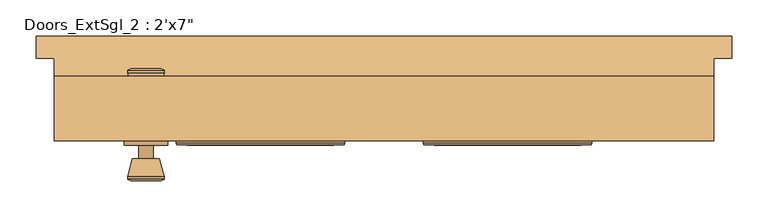
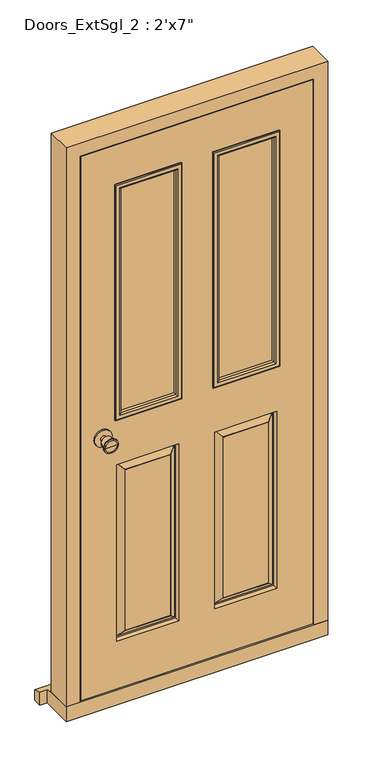
"""IFC4 building model written with IfcOpenShell, lengths in millimetres: door geometry."""

from ifc_helpers import new_model, si_unit, point, frame, frame_2d, origin, place, context, project, spatial, polyline, circle_curve, ellipse_curve, trimmed, segment, composite_curve, outline, extrude, faceted_brep, source, transform, mapped, element, save
from ifc_brep_helpers import plane_surface, cylinder_surface, revolved_surface, advanced_brep


def door_2817e3e8(model_context):
    return source(origin(), model_context, "Body", "SolidModel", [
        advanced_brep(
        [(-328.5, -18.4, 1000.0), (-318.5, -18.4, 1000.0), (-338.5, -18.4, 1000.0), (-308.0241324, -67.4, 1000.0), (-328.5, -67.4, 1000.0), (-348.9758676, -67.4, 1000.0), (-303.5, -65.5721319, 1000.0), (-353.5, -65.5721319, 1000.0), (-303.5, -62.1084537, 1000.0), (-353.5, -62.1084537, 1000.0), (-309.863764, -37.4, 1000.0), (-347.136236, -37.4, 1000.0), (-318.5, -37.4, 1000.0), (-338.5, -37.4, 1000.0)],
        [
            (0, 1),
            (1, 2, circle_curve(frame((-328.5, -18.4, 1000.0), z_axis=(0.0, 1.0, 0.0), x_axis=(-1.0, 0.0, 0.0)), 10.0)),
            (2, 0),
            (2, 1, circle_curve(frame((-328.5, -18.4, 1000.0), z_axis=(0.0, 1.0, 0.0), x_axis=(-1.0, 0.0, 0.0)), 10.0)),
            (3, 4),
            (4, 5),
            (5, 3, circle_curve(frame((-328.5, -67.4, 1000.0), z_axis=(0.0, -1.0, 0.0), x_axis=(-1.0, 0.0, 0.0)), 20.4758676)),
            (3, 5, circle_curve(frame((-328.5, -67.4, 1000.0), z_axis=(0.0, -1.0, 0.0), x_axis=(-1.0, 0.0, 0.0)), 20.4758676)),
            (6, 3),
            (5, 7),
            (7, 6, circle_curve(frame((-328.5, -65.5721319, 1000.0), z_axis=(0.0, -1.0, 0.0), x_axis=(-1.0, 0.0, 0.0)), 25.0)),
            (6, 7, circle_curve(frame((-328.5, -65.5721319, 1000.0), z_axis=(0.0, -1.0, 0.0), x_axis=(-1.0, 0.0, 0.0)), 25.0)),
            (8, 6),
            (7, 9),
            (9, 8, circle_curve(frame((-328.5, -62.1084537, 1000.0), z_axis=(0.0, -1.0, 0.0), x_axis=(-1.0, 0.0, 0.0)), 25.0)),
            (8, 9, circle_curve(frame((-328.5, -62.1084537, 1000.0), z_axis=(0.0, -1.0, 0.0), x_axis=(-1.0, 0.0, 0.0)), 25.0)),
            (10, 8),
            (9, 11),
            (11, 10, circle_curve(frame((-328.5, -37.4, 1000.0), z_axis=(0.0, -1.0, 0.0), x_axis=(-1.0, 0.0, 0.0)), 18.636236)),
            (10, 11, circle_curve(frame((-328.5, -37.4, 1000.0), z_axis=(0.0, -1.0, 0.0), x_axis=(-1.0, 0.0, 0.0)), 18.636236)),
            (12, 10),
            (11, 13),
            (13, 12, circle_curve(frame((-328.5, -37.4, 1000.0), z_axis=(0.0, -1.0, 0.0), x_axis=(-1.0, 0.0, 0.0)), 10.0)),
            (12, 13, circle_curve(frame((-328.5, -37.4, 1000.0), z_axis=(0.0, -1.0, 0.0), x_axis=(-1.0, 0.0, 0.0)), 10.0)),
            (1, 12),
            (13, 2),
        ],
        [
            plane_surface(frame((-328.5, -18.4, 1000.0), z_axis=(0.0, 1.0, 0.0), x_axis=(-1.0, 0.0, 0.0))),
            plane_surface(frame((-328.5, -67.4, 1000.0), z_axis=(0.0, -1.0, 0.0), x_axis=(-1.0, 0.0, 0.0))),
            revolved_surface(polyline([(-348.9758676, -67.4, 1000.0), (-353.5, -65.5721319, 1000.0)]), (-328.5, -18.4, 1000.0), (0.0, 1.0, 0.0)),
            cylinder_surface(frame((-328.5, -18.4, 1000.0), z_axis=(0.0, 1.0, 0.0), x_axis=(-1.0, 0.0, 0.0)), 25.0),
            revolved_surface(polyline([(-353.5, -62.1084537, 1000.0), (-347.136236, -37.4, 1000.0)]), (-328.5, -18.4, 1000.0), (0.0, 1.0, 0.0)),
            plane_surface(frame((-328.5, -37.4, 1000.0), z_axis=(0.0, 1.0, 0.0), x_axis=(-1.0, 0.0, 0.0))),
            cylinder_surface(frame((-328.5, -18.4, 1000.0), z_axis=(0.0, 1.0, 0.0), x_axis=(-1.0, 0.0, 0.0)), 10.0),
        ],
        [
            (0, [[1, 2, 3]]),
            (0, [[-3, 4, -1]]),
            (1, [[5, 6, 7]]),
            (1, [[-6, -5, 8]]),
            (2, [[9, -7, 10, 11]]),
            (2, [[-10, -8, -9, 12]]),
            (3, [[13, -11, 14, 15]]),
            (3, [[-14, -12, -13, 16]]),
            (4, [[17, -15, 18, 19]]),
            (4, [[-18, -16, -17, 20]]),
            (5, [[21, -19, 22, 23]]),
            (5, [[-22, -20, -21, 24]]),
            (6, [[25, -23, 26, -2]]),
            (6, [[-26, -24, -25, -4]]),
        ],
    ),
        extrude(outline(composite_curve([segment(trimmed(circle_curve(frame_2d((1000.0, -328.5)), 30.0), [point((1000.0, -358.5))], [point((1000.0, -298.5))], False, "CARTESIAN"), True, "CONTINUOUS"), segment(trimmed(circle_curve(frame_2d((1000.0, -328.5)), 30.0), [point((1000.0, -298.5))], [point((1000.0, -358.5))], False, "CARTESIAN"), True, "CONTINUOUS")], self_intersect=False)), frame((0.0, -18.4, 0.0), z_axis=(0.0, 1.0, 0.0), x_axis=(0.0, 0.0, 1.0)), (0.0, 0.0, 1.0), 6.0),
        advanced_brep(
        [(-328.5, 37.6, 1000.0), (-338.5, 37.6, 1000.0), (-318.5, 37.6, 1000.0), (-308.0241324, 86.6, 1000.0), (-348.9758676, 86.6, 1000.0), (-328.5, 86.6, 1000.0), (-303.5, 84.7721319, 1000.0), (-353.5, 84.7721319, 1000.0), (-303.5, 81.3084537, 1000.0), (-353.5, 81.3084537, 1000.0), (-309.863764, 56.6, 1000.0), (-347.136236, 56.6, 1000.0), (-318.5, 56.6, 1000.0), (-338.5, 56.6, 1000.0)],
        [
            (0, 1),
            (1, 2, circle_curve(frame((-328.5, 37.6, 1000.0), z_axis=(0.0, -1.0, 0.0), x_axis=(-1.0, 0.0, 0.0)), 10.0)),
            (2, 0),
            (2, 1, circle_curve(frame((-328.5, 37.6, 1000.0), z_axis=(0.0, -1.0, 0.0), x_axis=(-1.0, 0.0, 0.0)), 10.0)),
            (3, 4, circle_curve(frame((-328.5, 86.6, 1000.0), z_axis=(0.0, 1.0, 0.0), x_axis=(-1.0, 0.0, 0.0)), 20.4758676)),
            (4, 5),
            (5, 3),
            (4, 3, circle_curve(frame((-328.5, 86.6, 1000.0), z_axis=(0.0, 1.0, 0.0), x_axis=(-1.0, 0.0, 0.0)), 20.4758676)),
            (6, 7, circle_curve(frame((-328.5, 84.7721319, 1000.0), z_axis=(0.0, 1.0, 0.0), x_axis=(-1.0, 0.0, 0.0)), 25.0)),
            (7, 4),
            (3, 6),
            (7, 6, circle_curve(frame((-328.5, 84.7721319, 1000.0), z_axis=(0.0, 1.0, 0.0), x_axis=(-1.0, 0.0, 0.0)), 25.0)),
            (8, 9, circle_curve(frame((-328.5, 81.3084537, 1000.0), z_axis=(0.0, 1.0, 0.0), x_axis=(-1.0, 0.0, 0.0)), 25.0)),
            (9, 7),
            (6, 8),
            (9, 8, circle_curve(frame((-328.5, 81.3084537, 1000.0), z_axis=(0.0, 1.0, 0.0), x_axis=(-1.0, 0.0, 0.0)), 25.0)),
            (10, 11, circle_curve(frame((-328.5, 56.6, 1000.0), z_axis=(0.0, 1.0, 0.0), x_axis=(-1.0, 0.0, 0.0)), 18.636236)),
            (11, 9),
            (8, 10),
            (11, 10, circle_curve(frame((-328.5, 56.6, 1000.0), z_axis=(0.0, 1.0, 0.0), x_axis=(-1.0, 0.0, 0.0)), 18.636236)),
            (12, 13, circle_curve(frame((-328.5, 56.6, 1000.0), z_axis=(0.0, 1.0, 0.0), x_axis=(-1.0, 0.0, 0.0)), 10.0)),
            (13, 11),
            (10, 12),
            (13, 12, circle_curve(frame((-328.5, 56.6, 1000.0), z_axis=(0.0, 1.0, 0.0), x_axis=(-1.0, 0.0, 0.0)), 10.0)),
            (1, 13),
            (12, 2),
        ],
        [
            plane_surface(frame((-328.5, 37.6, 1000.0), z_axis=(0.0, -1.0, 0.0), x_axis=(-1.0, 0.0, 0.0))),
            plane_surface(frame((-328.5, 86.6, 1000.0), z_axis=(0.0, 1.0, 0.0), x_axis=(-1.0, 0.0, 0.0))),
            revolved_surface(polyline([(-348.9758676, 86.6, 1000.0), (-353.5, 84.7721319, 1000.0)]), (-328.5, 37.6, 1000.0), (0.0, -1.0, 0.0)),
            cylinder_surface(frame((-328.5, 37.6, 1000.0), z_axis=(0.0, -1.0, 0.0), x_axis=(-1.0, 0.0, 0.0)), 25.0),
            revolved_surface(polyline([(-353.5, 81.3084537, 1000.0), (-347.136236, 56.6, 1000.0)]), (-328.5, 37.6, 1000.0), (0.0, -1.0, 0.0)),
            plane_surface(frame((-328.5, 56.6, 1000.0), z_axis=(0.0, -1.0, 0.0), x_axis=(-1.0, 0.0, 0.0))),
            cylinder_surface(frame((-328.5, 37.6, 1000.0), z_axis=(0.0, -1.0, 0.0), x_axis=(-1.0, 0.0, 0.0)), 10.0),
        ],
        [
            (0, [[1, 2, 3]]),
            (0, [[-3, 4, -1]]),
            (1, [[5, 6, 7]]),
            (1, [[8, -7, -6]]),
            (2, [[9, 10, -5, 11]]),
            (2, [[12, -11, -8, -10]]),
            (3, [[13, 14, -9, 15]]),
            (3, [[16, -15, -12, -14]]),
            (4, [[17, 18, -13, 19]]),
            (4, [[20, -19, -16, -18]]),
            (5, [[21, 22, -17, 23]]),
            (5, [[24, -23, -20, -22]]),
            (6, [[-2, 25, -21, 26]]),
            (6, [[-4, -26, -24, -25]]),
        ],
    ),
        extrude(outline(composite_curve([segment(trimmed(circle_curve(frame_2d((1000.0, -328.5)), 30.0), [point((1000.0, -358.5))], [point((1000.0, -298.5))], False, "CARTESIAN"), True, "CONTINUOUS"), segment(trimmed(circle_curve(frame_2d((1000.0, -328.5)), 30.0), [point((1000.0, -298.5))], [point((1000.0, -358.5))], False, "CARTESIAN"), True, "CONTINUOUS")], self_intersect=False)), frame((0.0, 31.6, 0.0), z_axis=(0.0, 1.0, 0.0), x_axis=(0.0, 0.0, 1.0)), (0.0, 0.0, 1.0), 6.0),
        faceted_brep([(384.5, 76.6, 54.5), (455.0, 76.6, 54.5), (455.0, -12.4, 54.5), (406.5, -12.4, 54.5), (406.5, 34.6, 54.5), (384.5, 34.6, 54.5), (384.5, 76.6, 2039.5), (-384.5, 76.6, 2039.5), (-384.5, 76.6, 54.5), (-455.0, 76.6, 54.5), (-455.0, 76.6, 2110.0), (455.0, 76.6, 2110.0), (455.0, -12.4, 2110.0), (-455.0, -12.4, 2110.0), (-455.0, -12.4, 54.5), (-406.5, -12.4, 54.5), (-406.5, -12.4, 2061.5), (406.5, -12.4, 2061.5), (406.5, 34.6, 2061.5), (-406.5, 34.6, 2061.5), (-406.5, 34.6, 54.5), (-384.5, 34.6, 54.5), (-384.5, 34.6, 2039.5), (384.5, 34.6, 2039.5)], [[[0, 1, 2, 3, 4, 5]], [[1, 0, 6, 7, 8, 9, 10, 11]], [[2, 1, 11, 12]], [[3, 2, 12, 13, 14, 15, 16, 17]], [[4, 3, 17, 18]], [[5, 4, 18, 19, 20, 21, 22, 23]], [[0, 5, 23, 6]], [[8, 7, 22, 21]], [[9, 8, 21, 20, 15, 14]], [[10, 9, 14, 13]], [[16, 15, 20, 19]], [[11, 10, 13, 12]], [[17, 16, 19, 18]], [[7, 6, 23, 22]]]),
        faceted_brep([(403.5, -12.4, 58.5), (403.5, -12.4, 2058.5), (-404.4250294, -12.4, 2058.5), (-404.4250294, -12.4, 58.5), (62.5, -12.4, 1058.5), (62.5, -12.4, 1908.5), (278.5, -12.4, 1908.5), (278.5, -12.4, 1058.5), (-278.5, -12.4, 1058.5), (-278.5, -12.4, 1908.5), (-62.5, -12.4, 1908.5), (-62.5, -12.4, 1058.5), (-62.5, -12.4, 883.5), (-62.5, -12.4, 233.5), (-278.5, -12.4, 233.5), (-278.5, -12.4, 883.5), (278.5, -12.4, 883.5), (278.5, -12.4, 233.5), (62.5, -12.4, 233.5), (62.5, -12.4, 883.5), (-92.5, -12.4, 263.5), (-92.5, -12.4, 853.5), (-248.5, -12.4, 853.5), (-248.5, -12.4, 263.5), (248.5, -12.4, 263.5), (248.5, -12.4, 853.5), (92.5, -12.4, 853.5), (92.5, -12.4, 263.5), (403.5, 31.6, 58.5), (-404.4250294, 31.6, 58.5), (-404.4250294, 31.6, 2058.5), (403.5, 31.6, 2058.5), (62.5, 31.6, 1058.5), (278.5, 31.6, 1058.5), (278.5, 31.6, 1908.5), (62.5, 31.6, 1908.5), (-278.5, 31.6, 1058.5), (-62.5, 31.6, 1058.5), (-62.5, 31.6, 1908.5), (-278.5, 31.6, 1908.5), (62.5, 31.6, 883.5), (62.5, 31.6, 233.5), (278.5, 31.6, 233.5), (278.5, 31.6, 883.5), (-278.5, 31.6, 883.5), (-278.5, 31.6, 233.5), (-62.5, 31.6, 233.5), (-62.5, 31.6, 883.5), (92.5, 31.6, 263.5), (92.5, 31.6, 853.5), (248.5, 31.6, 853.5), (248.5, 31.6, 263.5), (-248.5, 31.6, 263.5), (-248.5, 31.6, 853.5), (-92.5, 31.6, 853.5), (-92.5, 31.6, 263.5), (65.5, 16.6, 880.5), (65.5, 16.6, 236.5), (90.5, 30.6, 855.5), (90.5, 30.6, 261.5), (70.5, 16.6, 241.5), (70.5, 16.6, 875.5), (92.5, 30.6, 263.5), (92.5, 30.6, 853.5), (275.5, 16.6, 236.5), (250.5, 30.6, 261.5), (270.5, 16.6, 241.5), (248.5, 30.6, 263.5), (275.5, 16.6, 880.5), (250.5, 30.6, 855.5), (270.5, 16.6, 875.5), (248.5, 30.6, 853.5), (-275.5, 16.6, 880.5), (-275.5, 16.6, 236.5), (-250.5, 30.6, 855.5), (-250.5, 30.6, 261.5), (-270.5, 16.6, 241.5), (-270.5, 16.6, 875.5), (-248.5, 30.6, 263.5), (-248.5, 30.6, 853.5), (-65.5, 16.6, 236.5), (-90.5, 30.6, 261.5), (-70.5, 16.6, 241.5), (-92.5, 30.6, 263.5), (-65.5, 16.6, 880.5), (-90.5, 30.6, 855.5), (-70.5, 16.6, 875.5), (-92.5, 30.6, 853.5), (-92.5, -11.4, 263.5), (-92.5, -11.4, 853.5), (-70.5, 2.6, 241.5), (-70.5, 2.6, 875.5), (-90.5, -11.4, 855.5), (-90.5, -11.4, 261.5), (-65.5, 2.6, 880.5), (-65.5, 2.6, 236.5), (-248.5, -11.4, 853.5), (-270.5, 2.6, 875.5), (-250.5, -11.4, 855.5), (-275.5, 2.6, 880.5), (-248.5, -11.4, 263.5), (-270.5, 2.6, 241.5), (-250.5, -11.4, 261.5), (-275.5, 2.6, 236.5), (275.5, 2.6, 880.5), (275.5, 2.6, 236.5), (250.5, -11.4, 855.5), (250.5, -11.4, 261.5), (270.5, 2.6, 241.5), (270.5, 2.6, 875.5), (248.5, -11.4, 263.5), (248.5, -11.4, 853.5), (65.5, 2.6, 236.5), (90.5, -11.4, 261.5), (70.5, 2.6, 241.5), (92.5, -11.4, 263.5), (65.5, 2.6, 880.5), (90.5, -11.4, 855.5), (70.5, 2.6, 875.5), (92.5, -11.4, 853.5)], [[[0, 1, 2, 3], [4, 5, 6, 7], [8, 9, 10, 11], [12, 13, 14, 15], [16, 17, 18, 19]], [[20, 21, 22, 23]], [[24, 25, 26, 27]], [[28, 29, 30, 31], [32, 33, 34, 35], [36, 37, 38, 39], [40, 41, 42, 43], [44, 45, 46, 47]], [[48, 49, 50, 51]], [[52, 53, 54, 55]], [[1, 0, 28, 31]], [[2, 1, 31, 30]], [[3, 2, 30, 29]], [[0, 3, 29, 28]], [[5, 4, 32, 35]], [[6, 5, 35, 34]], [[7, 6, 34, 33]], [[4, 7, 33, 32]], [[9, 8, 36, 39]], [[10, 9, 39, 38]], [[11, 10, 38, 37]], [[8, 11, 37, 36]], [[56, 57, 41, 40]], [[58, 59, 60, 61]], [[48, 62, 63, 49]], [[41, 57, 64, 42]], [[60, 59, 65, 66]], [[62, 48, 51, 67]], [[42, 64, 68, 43]], [[66, 65, 69, 70]], [[67, 51, 50, 71]], [[56, 40, 43, 68]], [[57, 56, 68, 64], [61, 60, 66, 70]], [[58, 61, 70, 69]], [[59, 58, 69, 65], [63, 62, 67, 71]], [[49, 63, 71, 50]], [[72, 73, 45, 44]], [[74, 75, 76, 77]], [[52, 78, 79, 53]], [[45, 73, 80, 46]], [[76, 75, 81, 82]], [[78, 52, 55, 83]], [[46, 80, 84, 47]], [[82, 81, 85, 86]], [[83, 55, 54, 87]], [[72, 44, 47, 84]], [[73, 72, 84, 80], [77, 76, 82, 86]], [[74, 77, 86, 85]], [[75, 74, 85, 81], [79, 78, 83, 87]], [[53, 79, 87, 54]], [[88, 89, 21, 20]], [[90, 91, 92, 93]], [[12, 94, 95, 13]], [[21, 89, 96, 22]], [[92, 91, 97, 98]], [[94, 12, 15, 99]], [[22, 96, 100, 23]], [[98, 97, 101, 102]], [[99, 15, 14, 103]], [[88, 20, 23, 100]], [[93, 92, 98, 102], [89, 88, 100, 96]], [[90, 93, 102, 101]], [[95, 94, 99, 103], [91, 90, 101, 97]], [[13, 95, 103, 14]], [[104, 105, 17, 16]], [[106, 107, 108, 109]], [[24, 110, 111, 25]], [[17, 105, 112, 18]], [[108, 107, 113, 114]], [[110, 24, 27, 115]], [[18, 112, 116, 19]], [[114, 113, 117, 118]], [[115, 27, 26, 119]], [[104, 16, 19, 116]], [[105, 104, 116, 112], [109, 108, 114, 118]], [[106, 109, 118, 117]], [[107, 106, 117, 113], [111, 110, 115, 119]], [[25, 111, 119, 26]]]),
        faceted_brep([(480.0, 131.6, 0.0), (480.0, 131.6, 38.5947221), (480.0, 101.6, 47.2703282), (480.0, 101.6, 0.0), (-480.0, 131.6, 38.5947221), (-480.0, 131.6, 0.0), (-480.0, 101.6, 0.0), (-480.0, 101.6, 47.2703282), (455.0, 101.6, 0.0), (455.0, -12.4, 0.0), (-455.0, -12.4, 0.0), (-455.0, 101.6, 0.0), (-455.0, 101.6, 47.2703282), (-455.0, 76.6, 54.5), (455.0, 76.6, 54.5), (455.0, 101.6, 47.2703282), (-455.0, -12.4, 54.5), (455.0, -12.4, 54.5)], [[[0, 1, 2, 3]], [[4, 5, 6, 7]], [[5, 0, 3, 8, 9, 10, 11, 6]], [[1, 0, 5, 4]], [[1, 4, 7, 12, 13, 14, 15, 2]], [[13, 16, 17, 14]], [[16, 10, 9, 17]], [[12, 11, 10, 16, 13]], [[11, 12, 7, 6]], [[8, 15, 14, 17, 9]], [[15, 8, 3, 2]]]),
        extrude(outline(polyline([(278.5, -2.4), (62.5, -2.4), (62.5, 21.6), (278.5, 21.6), (278.5, -2.4)])), frame((0.0, 0.0, 1058.5), z_axis=(0.0, 0.0, 1.0), x_axis=(1.0, 0.0, 0.0)), (0.0, 0.0, 1.0), 850.0),
        extrude(outline(polyline([(-62.5, -2.4), (-278.5, -2.4), (-278.5, 21.6), (-62.5, 21.6), (-62.5, -2.4)])), frame((0.0, 0.0, 1058.5), z_axis=(0.0, 0.0, 1.0), x_axis=(1.0, 0.0, 0.0)), (0.0, 0.0, 1.0), 850.0),
        advanced_brep(
        [(286.5, 35.6, 1916.5), (286.5, 31.6, 1916.5), (286.5, 31.6, 1050.5), (286.5, 35.6, 1050.5), (284.5, 37.6, 1914.5), (284.5, 37.6, 1052.5), (266.5, 32.6, 1896.5), (271.5, 37.6, 1901.5), (271.5, 37.6, 1065.5), (266.5, 32.6, 1070.5), (266.5, 21.6, 1896.5), (266.5, 21.6, 1070.5), (278.5, 31.6, 1908.5), (278.5, 21.6, 1908.5), (278.5, 21.6, 1058.5), (278.5, 31.6, 1058.5), (54.5, 31.6, 1050.5), (54.5, 35.6, 1050.5), (56.5, 37.6, 1052.5), (69.5, 37.6, 1065.5), (74.5, 32.6, 1070.5), (74.5, 21.6, 1070.5), (62.5, 21.6, 1058.5), (62.5, 31.6, 1058.5), (54.5, 31.6, 1916.5), (54.5, 35.6, 1916.5), (56.5, 37.6, 1914.5), (69.5, 37.6, 1901.5), (74.5, 32.6, 1896.5), (74.5, 21.6, 1896.5), (62.5, 21.6, 1908.5), (62.5, 31.6, 1908.5)],
        [
            (0, 1),
            (1, 2),
            (2, 3),
            (3, 0),
            (4, 0, ellipse_curve(frame((284.5, 35.6, 1914.5), z_axis=(0.7071067811865475, 0.0, -0.7071067811865475), x_axis=(0.7071067811865474, 0.0, 0.7071067811865476)), 2.8284271, 2.0)),
            (3, 5, ellipse_curve(frame((284.5, 35.6, 1052.5), z_axis=(0.7071067811865475, 0.0, 0.7071067811865475), x_axis=(-0.7071067811865474, 0.0, 0.7071067811865476)), 2.8284271, 2.0)),
            (5, 4),
            (6, 7, ellipse_curve(frame((271.5, 32.6, 1901.5), z_axis=(0.7071067811865475, 0.0, -0.7071067811865475), x_axis=(0.7071067811865474, 0.0, 0.7071067811865476)), 7.0710678, 5.0)),
            (7, 8),
            (8, 9, ellipse_curve(frame((271.5, 32.6, 1065.5), z_axis=(0.7071067811865475, 0.0, 0.7071067811865475), x_axis=(-0.7071067811865474, 0.0, 0.7071067811865476)), 7.0710678, 5.0)),
            (9, 6),
            (10, 6),
            (9, 11),
            (11, 10),
            (12, 13),
            (13, 14),
            (14, 15),
            (15, 12),
            (2, 16),
            (16, 17),
            (17, 3),
            (17, 18, ellipse_curve(frame((56.5, 35.6, 1052.5), z_axis=(0.7071067811865475, 0.0, -0.7071067811865475), x_axis=(0.7071067811865476, 0.0, 0.7071067811865474)), 2.8284271, 2.0)),
            (18, 5),
            (8, 19),
            (19, 20, ellipse_curve(frame((69.5, 32.6, 1065.5), z_axis=(0.7071067811865475, 0.0, -0.7071067811865475), x_axis=(0.7071067811865476, 0.0, 0.7071067811865474)), 7.0710678, 5.0)),
            (20, 9),
            (20, 21),
            (21, 11),
            (14, 22),
            (22, 23),
            (23, 15),
            (16, 24),
            (24, 25),
            (25, 17),
            (25, 26, ellipse_curve(frame((56.5, 35.6, 1914.5), z_axis=(-0.7071067811865475, 0.0, -0.7071067811865475), x_axis=(0.7071067811865474, 0.0, -0.7071067811865476)), 2.8284271, 2.0)),
            (26, 18),
            (19, 27),
            (27, 28, ellipse_curve(frame((69.5, 32.6, 1901.5), z_axis=(-0.7071067811865475, 0.0, -0.7071067811865475), x_axis=(0.7071067811865474, 0.0, -0.7071067811865476)), 7.0710678, 5.0)),
            (28, 20),
            (28, 29),
            (29, 21),
            (22, 30),
            (30, 31),
            (31, 23),
            (24, 1),
            (0, 25),
            (4, 26),
            (7, 27),
            (6, 28),
            (10, 29),
            (13, 30),
            (12, 31),
        ],
        [
            plane_surface(frame((286.5, 31.6, 1916.5), z_axis=(1.0, 0.0, 0.0), x_axis=(0.0, 0.0, -1.0))),
            cylinder_surface(frame((284.5, 35.6, 1908.5), z_axis=(0.0, 0.0, 1.0), x_axis=(1.0, 0.0, 0.0)), 2.0),
            cylinder_surface(frame((271.5, 32.6, 1908.5), z_axis=(0.0, 0.0, 1.0), x_axis=(1.0, 0.0, 0.0)), 5.0),
            plane_surface(frame((266.5, 32.6, 1896.5), z_axis=(-1.0, 0.0, 0.0), x_axis=(0.0, 0.0, -1.0))),
            plane_surface(frame((278.5, 21.6, 1908.5), z_axis=(1.0, 0.0, 0.0), x_axis=(0.0, 0.0, -1.0))),
            plane_surface(frame((286.5, 31.6, 1050.5), z_axis=(0.0, 0.0, -1.0), x_axis=(-1.0, 0.0, 0.0))),
            cylinder_surface(frame((278.5, 35.6, 1052.5), z_axis=(1.0, 0.0, 0.0), x_axis=(0.0, 0.0, -1.0)), 2.0),
            cylinder_surface(frame((278.5, 32.6, 1065.5), z_axis=(1.0, 0.0, 0.0), x_axis=(0.0, 0.0, -1.0)), 5.0),
            plane_surface(frame((266.5, 32.6, 1070.5), z_axis=(0.0, 0.0, 1.0), x_axis=(-1.0, 0.0, 0.0))),
            plane_surface(frame((278.5, 21.6, 1058.5), z_axis=(0.0, 0.0, -1.0), x_axis=(-1.0, 0.0, 0.0))),
            plane_surface(frame((54.5, 31.6, 1050.5), z_axis=(-1.0, 0.0, 0.0), x_axis=(0.0, 0.0, 1.0))),
            cylinder_surface(frame((56.5, 35.6, 1058.5), z_axis=(0.0, 0.0, -1.0), x_axis=(-1.0, 0.0, 0.0)), 2.0),
            cylinder_surface(frame((69.5, 32.6, 1058.5), z_axis=(0.0, 0.0, -1.0), x_axis=(-1.0, 0.0, 0.0)), 5.0),
            plane_surface(frame((74.5, 32.6, 1070.5), z_axis=(1.0, 0.0, 0.0), x_axis=(0.0, 0.0, 1.0))),
            plane_surface(frame((62.5, 21.6, 1058.5), z_axis=(-1.0, 0.0, 0.0), x_axis=(0.0, 0.0, 1.0))),
            plane_surface(frame((54.5, 31.6, 1916.5), z_axis=(0.0, 0.0, 1.0), x_axis=(1.0, 0.0, 0.0))),
            cylinder_surface(frame((62.5, 35.6, 1914.5), z_axis=(-1.0, 0.0, 0.0), x_axis=(0.0, 0.0, 1.0)), 2.0),
            plane_surface(frame((56.5, 37.6, 1914.5), z_axis=(0.0, 1.0, 0.0), x_axis=(1.0, 0.0, 0.0))),
            cylinder_surface(frame((62.5, 32.6, 1901.5), z_axis=(-1.0, 0.0, 0.0), x_axis=(0.0, 0.0, 1.0)), 5.0),
            plane_surface(frame((74.5, 32.6, 1896.5), z_axis=(0.0, 0.0, -1.0), x_axis=(1.0, 0.0, 0.0))),
            plane_surface(frame((74.5, 21.6, 1896.5), z_axis=(0.0, -1.0, 0.0), x_axis=(1.0, 0.0, 0.0))),
            plane_surface(frame((62.5, 21.6, 1908.5), z_axis=(0.0, 0.0, 1.0), x_axis=(1.0, 0.0, 0.0))),
            plane_surface(frame((62.5, 31.6, 1908.5), z_axis=(0.0, -1.0, 0.0), x_axis=(1.0, 0.0, 0.0))),
        ],
        [
            (0, [[1, 2, 3, 4]]),
            (1, [[5, -4, 6, 7]]),
            (2, [[8, 9, 10, 11]]),
            (3, [[12, -11, 13, 14]]),
            (4, [[15, 16, 17, 18]]),
            (5, [[-3, 19, 20, 21]]),
            (6, [[-6, -21, 22, 23]]),
            (7, [[-10, 24, 25, 26]]),
            (8, [[-13, -26, 27, 28]]),
            (9, [[-17, 29, 30, 31]]),
            (10, [[-20, 32, 33, 34]]),
            (11, [[-22, -34, 35, 36]]),
            (12, [[-25, 37, 38, 39]]),
            (13, [[-27, -39, 40, 41]]),
            (14, [[-30, 42, 43, 44]]),
            (15, [[-33, 45, -1, 46]]),
            (16, [[-35, -46, -5, 47]]),
            (17, [[-23, -36, -47, -7], [48, -37, -24, -9]]),
            (18, [[-38, -48, -8, 49]]),
            (19, [[-40, -49, -12, 50]]),
            (20, [[51, -42, -29, -16], [-28, -41, -50, -14]]),
            (21, [[-43, -51, -15, 52]]),
            (22, [[-45, -32, -19, -2], [-31, -44, -52, -18]]),
        ],
    ),
        advanced_brep(
        [(-54.5, 35.6, 1050.5), (-54.5, 31.6, 1050.5), (-286.5, 31.6, 1050.5), (-286.5, 35.6, 1050.5), (-56.5, 37.6, 1052.5), (-284.5, 37.6, 1052.5), (-74.5, 32.6, 1070.5), (-69.5, 37.6, 1065.5), (-271.5, 37.6, 1065.5), (-266.5, 32.6, 1070.5), (-74.5, 21.6, 1070.5), (-266.5, 21.6, 1070.5), (-62.5, 31.6, 1058.5), (-62.5, 21.6, 1058.5), (-278.5, 21.6, 1058.5), (-278.5, 31.6, 1058.5), (-286.5, 31.6, 1916.5), (-286.5, 35.6, 1916.5), (-284.5, 37.6, 1914.5), (-271.5, 37.6, 1901.5), (-266.5, 32.6, 1896.5), (-266.5, 21.6, 1896.5), (-278.5, 21.6, 1908.5), (-278.5, 31.6, 1908.5), (-54.5, 31.6, 1916.5), (-54.5, 35.6, 1916.5), (-56.5, 37.6, 1914.5), (-69.5, 37.6, 1901.5), (-74.5, 32.6, 1896.5), (-74.5, 21.6, 1896.5), (-62.5, 21.6, 1908.5), (-62.5, 31.6, 1908.5)],
        [
            (0, 1),
            (1, 2),
            (2, 3),
            (3, 0),
            (4, 0, ellipse_curve(frame((-56.5, 35.6, 1052.5), z_axis=(-0.7071067811865475, 0.0, -0.7071067811865475), x_axis=(0.7071067811865476, 0.0, -0.7071067811865474)), 2.8284271, 2.0)),
            (3, 5, ellipse_curve(frame((-284.5, 35.6, 1052.5), z_axis=(0.7071067811865475, 0.0, -0.7071067811865475), x_axis=(0.7071067811865476, 0.0, 0.7071067811865474)), 2.8284271, 2.0)),
            (5, 4),
            (6, 7, ellipse_curve(frame((-69.5, 32.6, 1065.5), z_axis=(-0.7071067811865475, 0.0, -0.7071067811865475), x_axis=(0.7071067811865476, 0.0, -0.7071067811865474)), 7.0710678, 5.0)),
            (7, 8),
            (8, 9, ellipse_curve(frame((-271.5, 32.6, 1065.5), z_axis=(0.7071067811865475, 0.0, -0.7071067811865475), x_axis=(0.7071067811865476, 0.0, 0.7071067811865474)), 7.0710678, 5.0)),
            (9, 6),
            (10, 6),
            (9, 11),
            (11, 10),
            (12, 13),
            (13, 14),
            (14, 15),
            (15, 12),
            (2, 16),
            (16, 17),
            (17, 3),
            (17, 18, ellipse_curve(frame((-284.5, 35.6, 1914.5), z_axis=(-0.7071067811865475, 0.0, -0.7071067811865475), x_axis=(0.7071067811865474, 0.0, -0.7071067811865476)), 2.8284271, 2.0)),
            (18, 5),
            (8, 19),
            (19, 20, ellipse_curve(frame((-271.5, 32.6, 1901.5), z_axis=(-0.7071067811865475, 0.0, -0.7071067811865475), x_axis=(0.7071067811865474, 0.0, -0.7071067811865476)), 7.0710678, 5.0)),
            (20, 9),
            (20, 21),
            (21, 11),
            (14, 22),
            (22, 23),
            (23, 15),
            (16, 24),
            (24, 25),
            (25, 17),
            (25, 26, ellipse_curve(frame((-56.5, 35.6, 1914.5), z_axis=(-0.7071067811865475, 0.0, 0.7071067811865475), x_axis=(-0.7071067811865476, 0.0, -0.7071067811865474)), 2.8284271, 2.0)),
            (26, 18),
            (19, 27),
            (27, 28, ellipse_curve(frame((-69.5, 32.6, 1901.5), z_axis=(-0.7071067811865475, 0.0, 0.7071067811865475), x_axis=(-0.7071067811865476, 0.0, -0.7071067811865474)), 7.0710678, 5.0)),
            (28, 20),
            (28, 29),
            (29, 21),
            (22, 30),
            (30, 31),
            (31, 23),
            (24, 1),
            (0, 25),
            (4, 26),
            (7, 27),
            (6, 28),
            (10, 29),
            (13, 30),
            (12, 31),
        ],
        [
            plane_surface(frame((-54.5, 31.6, 1050.5), z_axis=(0.0, 0.0, -1.0), x_axis=(-1.0, 0.0, 0.0))),
            cylinder_surface(frame((-62.5, 35.6, 1052.5), z_axis=(1.0, 0.0, 0.0), x_axis=(0.0, 0.0, -1.0)), 2.0),
            cylinder_surface(frame((-62.5, 32.6, 1065.5), z_axis=(1.0, 0.0, 0.0), x_axis=(0.0, 0.0, -1.0)), 5.0),
            plane_surface(frame((-74.5, 32.6, 1070.5), z_axis=(0.0, 0.0, 1.0), x_axis=(-1.0, 0.0, 0.0))),
            plane_surface(frame((-62.5, 21.6, 1058.5), z_axis=(0.0, 0.0, -1.0), x_axis=(-1.0, 0.0, 0.0))),
            plane_surface(frame((-286.5, 31.6, 1050.5), z_axis=(-1.0, 0.0, 0.0), x_axis=(0.0, 0.0, 1.0))),
            cylinder_surface(frame((-284.5, 35.6, 1058.5), z_axis=(0.0, 0.0, -1.0), x_axis=(-1.0, 0.0, 0.0)), 2.0),
            cylinder_surface(frame((-271.5, 32.6, 1058.5), z_axis=(0.0, 0.0, -1.0), x_axis=(-1.0, 0.0, 0.0)), 5.0),
            plane_surface(frame((-266.5, 32.6, 1070.5), z_axis=(1.0, 0.0, 0.0), x_axis=(0.0, 0.0, 1.0))),
            plane_surface(frame((-278.5, 21.6, 1058.5), z_axis=(-1.0, 0.0, 0.0), x_axis=(0.0, 0.0, 1.0))),
            plane_surface(frame((-286.5, 31.6, 1916.5), z_axis=(0.0, 0.0, 1.0), x_axis=(1.0, 0.0, 0.0))),
            cylinder_surface(frame((-278.5, 35.6, 1914.5), z_axis=(-1.0, 0.0, 0.0), x_axis=(0.0, 0.0, 1.0)), 2.0),
            cylinder_surface(frame((-278.5, 32.6, 1901.5), z_axis=(-1.0, 0.0, 0.0), x_axis=(0.0, 0.0, 1.0)), 5.0),
            plane_surface(frame((-266.5, 32.6, 1896.5), z_axis=(0.0, 0.0, -1.0), x_axis=(1.0, 0.0, 0.0))),
            plane_surface(frame((-278.5, 21.6, 1908.5), z_axis=(0.0, 0.0, 1.0), x_axis=(1.0, 0.0, 0.0))),
            plane_surface(frame((-54.5, 31.6, 1916.5), z_axis=(1.0, 0.0, 0.0), x_axis=(0.0, 0.0, -1.0))),
            cylinder_surface(frame((-56.5, 35.6, 1908.5), z_axis=(0.0, 0.0, 1.0), x_axis=(1.0, 0.0, 0.0)), 2.0),
            plane_surface(frame((-56.5, 37.6, 1914.5), z_axis=(0.0, 1.0, 0.0), x_axis=(0.0, 0.0, -1.0))),
            cylinder_surface(frame((-69.5, 32.6, 1908.5), z_axis=(0.0, 0.0, 1.0), x_axis=(1.0, 0.0, 0.0)), 5.0),
            plane_surface(frame((-74.5, 32.6, 1896.5), z_axis=(-1.0, 0.0, 0.0), x_axis=(0.0, 0.0, -1.0))),
            plane_surface(frame((-74.5, 21.6, 1896.5), z_axis=(0.0, -1.0, 0.0), x_axis=(0.0, 0.0, -1.0))),
            plane_surface(frame((-62.5, 21.6, 1908.5), z_axis=(1.0, 0.0, 0.0), x_axis=(0.0, 0.0, -1.0))),
            plane_surface(frame((-62.5, 31.6, 1908.5), z_axis=(0.0, -1.0, 0.0), x_axis=(0.0, 0.0, -1.0))),
        ],
        [
            (0, [[1, 2, 3, 4]]),
            (1, [[5, -4, 6, 7]]),
            (2, [[8, 9, 10, 11]]),
            (3, [[12, -11, 13, 14]]),
            (4, [[15, 16, 17, 18]]),
            (5, [[-3, 19, 20, 21]]),
            (6, [[-6, -21, 22, 23]]),
            (7, [[-10, 24, 25, 26]]),
            (8, [[-13, -26, 27, 28]]),
            (9, [[-17, 29, 30, 31]]),
            (10, [[-20, 32, 33, 34]]),
            (11, [[-22, -34, 35, 36]]),
            (12, [[-25, 37, 38, 39]]),
            (13, [[-27, -39, 40, 41]]),
            (14, [[-30, 42, 43, 44]]),
            (15, [[-33, 45, -1, 46]]),
            (16, [[-35, -46, -5, 47]]),
            (17, [[-23, -36, -47, -7], [48, -37, -24, -9]]),
            (18, [[-38, -48, -8, 49]]),
            (19, [[-40, -49, -12, 50]]),
            (20, [[51, -42, -29, -16], [-28, -41, -50, -14]]),
            (21, [[-43, -51, -15, 52]]),
            (22, [[-45, -32, -19, -2], [-31, -44, -52, -18]]),
        ],
    ),
        advanced_brep(
        [(-278.5, -2.4, 1908.5), (-278.5, -12.4, 1908.5), (-62.5, -12.4, 1908.5), (-62.5, -2.4, 1908.5), (-266.5, -13.4, 1896.5), (-266.5, -2.4, 1896.5), (-74.5, -2.4, 1896.5), (-74.5, -13.4, 1896.5), (-271.5, -18.4, 1901.5), (-69.5, -18.4, 1901.5), (-286.5, -16.4, 1916.5), (-284.5, -18.4, 1914.5), (-56.5, -18.4, 1914.5), (-54.5, -16.4, 1916.5), (-286.5, -12.4, 1916.5), (-54.5, -12.4, 1916.5), (-62.5, -12.4, 1058.5), (-62.5, -2.4, 1058.5), (-74.5, -2.4, 1070.5), (-74.5, -13.4, 1070.5), (-69.5, -18.4, 1065.5), (-56.5, -18.4, 1052.5), (-54.5, -16.4, 1050.5), (-54.5, -12.4, 1050.5), (-278.5, -12.4, 1058.5), (-278.5, -2.4, 1058.5), (-266.5, -2.4, 1070.5), (-266.5, -13.4, 1070.5), (-271.5, -18.4, 1065.5), (-284.5, -18.4, 1052.5), (-286.5, -16.4, 1050.5), (-286.5, -12.4, 1050.5)],
        [
            (0, 1),
            (1, 2),
            (2, 3),
            (3, 0),
            (4, 5),
            (5, 6),
            (6, 7),
            (7, 4),
            (8, 4, ellipse_curve(frame((-271.5, -13.4, 1901.5), z_axis=(0.7071067811865475, 0.0, 0.7071067811865475), x_axis=(-0.7071067811865476, 0.0, 0.7071067811865474)), 7.0710678, 5.0)),
            (7, 9, ellipse_curve(frame((-69.5, -13.4, 1901.5), z_axis=(-0.7071067811865475, 0.0, 0.7071067811865475), x_axis=(-0.7071067811865476, 0.0, -0.7071067811865474)), 7.0710678, 5.0)),
            (9, 8),
            (10, 11, ellipse_curve(frame((-284.5, -16.4, 1914.5), z_axis=(0.7071067811865475, 0.0, 0.7071067811865475), x_axis=(-0.7071067811865476, 0.0, 0.7071067811865474)), 2.8284271, 2.0)),
            (11, 12),
            (12, 13, ellipse_curve(frame((-56.5, -16.4, 1914.5), z_axis=(-0.7071067811865475, 0.0, 0.7071067811865475), x_axis=(-0.7071067811865476, 0.0, -0.7071067811865474)), 2.8284271, 2.0)),
            (13, 10),
            (14, 10),
            (13, 15),
            (15, 14),
            (2, 16),
            (16, 17),
            (17, 3),
            (6, 18),
            (18, 19),
            (19, 7),
            (19, 20, ellipse_curve(frame((-69.5, -13.4, 1065.5), z_axis=(0.7071067811865475, 0.0, 0.7071067811865475), x_axis=(-0.7071067811865474, 0.0, 0.7071067811865476)), 7.0710678, 5.0)),
            (20, 9),
            (12, 21),
            (21, 22, ellipse_curve(frame((-56.5, -16.4, 1052.5), z_axis=(0.7071067811865475, 0.0, 0.7071067811865475), x_axis=(-0.7071067811865474, 0.0, 0.7071067811865476)), 2.8284271, 2.0)),
            (22, 13),
            (22, 23),
            (23, 15),
            (16, 24),
            (24, 25),
            (25, 17),
            (18, 26),
            (26, 27),
            (27, 19),
            (27, 28, ellipse_curve(frame((-271.5, -13.4, 1065.5), z_axis=(0.7071067811865475, 0.0, -0.7071067811865475), x_axis=(0.7071067811865476, 0.0, 0.7071067811865474)), 7.0710678, 5.0)),
            (28, 20),
            (21, 29),
            (29, 30, ellipse_curve(frame((-284.5, -16.4, 1052.5), z_axis=(0.7071067811865475, 0.0, -0.7071067811865475), x_axis=(0.7071067811865476, 0.0, 0.7071067811865474)), 2.8284271, 2.0)),
            (30, 22),
            (30, 31),
            (31, 23),
            (31, 14),
            (1, 24),
            (0, 25),
            (5, 26),
            (4, 27),
            (8, 28),
            (11, 29),
            (10, 30),
        ],
        [
            plane_surface(frame((-278.5, -12.4, 1908.5), z_axis=(0.0, 0.0, 1.0), x_axis=(1.0, 0.0, 0.0))),
            plane_surface(frame((-266.5, -2.4, 1896.5), z_axis=(0.0, 0.0, -1.0), x_axis=(1.0, 0.0, 0.0))),
            cylinder_surface(frame((-278.5, -13.4, 1901.5), z_axis=(-1.0, 0.0, 0.0), x_axis=(0.0, 0.0, 1.0)), 5.0),
            cylinder_surface(frame((-278.5, -16.4, 1914.5), z_axis=(-1.0, 0.0, 0.0), x_axis=(0.0, 0.0, 1.0)), 2.0),
            plane_surface(frame((-286.5, -16.4, 1916.5), z_axis=(0.0, 0.0, 1.0), x_axis=(1.0, 0.0, 0.0))),
            plane_surface(frame((-62.5, -12.4, 1908.5), z_axis=(1.0, 0.0, 0.0), x_axis=(0.0, 0.0, -1.0))),
            plane_surface(frame((-74.5, -2.4, 1896.5), z_axis=(-1.0, 0.0, 0.0), x_axis=(0.0, 0.0, -1.0))),
            cylinder_surface(frame((-69.5, -13.4, 1908.5), z_axis=(0.0, 0.0, 1.0), x_axis=(1.0, 0.0, 0.0)), 5.0),
            cylinder_surface(frame((-56.5, -16.4, 1908.5), z_axis=(0.0, 0.0, 1.0), x_axis=(1.0, 0.0, 0.0)), 2.0),
            plane_surface(frame((-54.5, -16.4, 1916.5), z_axis=(1.0, 0.0, 0.0), x_axis=(0.0, 0.0, -1.0))),
            plane_surface(frame((-62.5, -12.4, 1058.5), z_axis=(0.0, 0.0, -1.0), x_axis=(-1.0, 0.0, 0.0))),
            plane_surface(frame((-74.5, -2.4, 1070.5), z_axis=(0.0, 0.0, 1.0), x_axis=(-1.0, 0.0, 0.0))),
            cylinder_surface(frame((-62.5, -13.4, 1065.5), z_axis=(1.0, 0.0, 0.0), x_axis=(0.0, 0.0, -1.0)), 5.0),
            cylinder_surface(frame((-62.5, -16.4, 1052.5), z_axis=(1.0, 0.0, 0.0), x_axis=(0.0, 0.0, -1.0)), 2.0),
            plane_surface(frame((-54.5, -16.4, 1050.5), z_axis=(0.0, 0.0, -1.0), x_axis=(-1.0, 0.0, 0.0))),
            plane_surface(frame((-286.5, -12.4, 1050.5), z_axis=(0.0, 1.0, 0.0), x_axis=(0.0, 0.0, 1.0))),
            plane_surface(frame((-278.5, -12.4, 1058.5), z_axis=(-1.0, 0.0, 0.0), x_axis=(0.0, 0.0, 1.0))),
            plane_surface(frame((-278.5, -2.4, 1058.5), z_axis=(0.0, 1.0, 0.0), x_axis=(0.0, 0.0, 1.0))),
            plane_surface(frame((-266.5, -2.4, 1070.5), z_axis=(1.0, 0.0, 0.0), x_axis=(0.0, 0.0, 1.0))),
            cylinder_surface(frame((-271.5, -13.4, 1058.5), z_axis=(0.0, 0.0, -1.0), x_axis=(-1.0, 0.0, 0.0)), 5.0),
            plane_surface(frame((-271.5, -18.4, 1065.5), z_axis=(0.0, -1.0, 0.0), x_axis=(0.0, 0.0, 1.0))),
            cylinder_surface(frame((-284.5, -16.4, 1058.5), z_axis=(0.0, 0.0, -1.0), x_axis=(-1.0, 0.0, 0.0)), 2.0),
            plane_surface(frame((-286.5, -16.4, 1050.5), z_axis=(-1.0, 0.0, 0.0), x_axis=(0.0, 0.0, 1.0))),
        ],
        [
            (0, [[1, 2, 3, 4]]),
            (1, [[5, 6, 7, 8]]),
            (2, [[9, -8, 10, 11]]),
            (3, [[12, 13, 14, 15]]),
            (4, [[16, -15, 17, 18]]),
            (5, [[-3, 19, 20, 21]]),
            (6, [[-7, 22, 23, 24]]),
            (7, [[-10, -24, 25, 26]]),
            (8, [[-14, 27, 28, 29]]),
            (9, [[-17, -29, 30, 31]]),
            (10, [[-20, 32, 33, 34]]),
            (11, [[-23, 35, 36, 37]]),
            (12, [[-25, -37, 38, 39]]),
            (13, [[-28, 40, 41, 42]]),
            (14, [[-30, -42, 43, 44]]),
            (15, [[-31, -44, 45, -18], [46, -32, -19, -2]]),
            (16, [[-33, -46, -1, 47]]),
            (17, [[-21, -34, -47, -4], [48, -35, -22, -6]]),
            (18, [[-36, -48, -5, 49]]),
            (19, [[-38, -49, -9, 50]]),
            (20, [[51, -40, -27, -13], [-26, -39, -50, -11]]),
            (21, [[-41, -51, -12, 52]]),
            (22, [[-43, -52, -16, -45]]),
        ],
    ),
        advanced_brep(
        [(62.5, -2.4, 1908.5), (62.5, -12.4, 1908.5), (278.5, -12.4, 1908.5), (278.5, -2.4, 1908.5), (74.5, -13.4, 1896.5), (74.5, -2.4, 1896.5), (266.5, -2.4, 1896.5), (266.5, -13.4, 1896.5), (69.5, -18.4, 1901.5), (271.5, -18.4, 1901.5), (54.5, -16.4, 1916.5), (56.5, -18.4, 1914.5), (284.5, -18.4, 1914.5), (286.5, -16.4, 1916.5), (54.5, -12.4, 1916.5), (286.5, -12.4, 1916.5), (278.5, -12.4, 1058.5), (278.5, -2.4, 1058.5), (266.5, -2.4, 1070.5), (266.5, -13.4, 1070.5), (271.5, -18.4, 1065.5), (284.5, -18.4, 1052.5), (286.5, -16.4, 1050.5), (286.5, -12.4, 1050.5), (62.5, -12.4, 1058.5), (62.5, -2.4, 1058.5), (74.5, -2.4, 1070.5), (74.5, -13.4, 1070.5), (69.5, -18.4, 1065.5), (56.5, -18.4, 1052.5), (54.5, -16.4, 1050.5), (54.5, -12.4, 1050.5)],
        [
            (0, 1),
            (1, 2),
            (2, 3),
            (3, 0),
            (4, 5),
            (5, 6),
            (6, 7),
            (7, 4),
            (8, 4, ellipse_curve(frame((69.5, -13.4, 1901.5), z_axis=(0.7071067811865475, 0.0, 0.7071067811865475), x_axis=(-0.7071067811865476, 0.0, 0.7071067811865474)), 7.0710678, 5.0)),
            (7, 9, ellipse_curve(frame((271.5, -13.4, 1901.5), z_axis=(-0.7071067811865475, 0.0, 0.7071067811865475), x_axis=(-0.7071067811865476, 0.0, -0.7071067811865474)), 7.0710678, 5.0)),
            (9, 8),
            (10, 11, ellipse_curve(frame((56.5, -16.4, 1914.5), z_axis=(0.7071067811865475, 0.0, 0.7071067811865475), x_axis=(-0.7071067811865476, 0.0, 0.7071067811865474)), 2.8284271, 2.0)),
            (11, 12),
            (12, 13, ellipse_curve(frame((284.5, -16.4, 1914.5), z_axis=(-0.7071067811865475, 0.0, 0.7071067811865475), x_axis=(-0.7071067811865476, 0.0, -0.7071067811865474)), 2.8284271, 2.0)),
            (13, 10),
            (14, 10),
            (13, 15),
            (15, 14),
            (2, 16),
            (16, 17),
            (17, 3),
            (6, 18),
            (18, 19),
            (19, 7),
            (19, 20, ellipse_curve(frame((271.5, -13.4, 1065.5), z_axis=(0.7071067811865475, 0.0, 0.7071067811865475), x_axis=(-0.7071067811865474, 0.0, 0.7071067811865476)), 7.0710678, 5.0)),
            (20, 9),
            (12, 21),
            (21, 22, ellipse_curve(frame((284.5, -16.4, 1052.5), z_axis=(0.7071067811865475, 0.0, 0.7071067811865475), x_axis=(-0.7071067811865474, 0.0, 0.7071067811865476)), 2.8284271, 2.0)),
            (22, 13),
            (22, 23),
            (23, 15),
            (16, 24),
            (24, 25),
            (25, 17),
            (18, 26),
            (26, 27),
            (27, 19),
            (27, 28, ellipse_curve(frame((69.5, -13.4, 1065.5), z_axis=(0.7071067811865475, 0.0, -0.7071067811865475), x_axis=(0.7071067811865476, 0.0, 0.7071067811865474)), 7.0710678, 5.0)),
            (28, 20),
            (21, 29),
            (29, 30, ellipse_curve(frame((56.5, -16.4, 1052.5), z_axis=(0.7071067811865475, 0.0, -0.7071067811865475), x_axis=(0.7071067811865476, 0.0, 0.7071067811865474)), 2.8284271, 2.0)),
            (30, 22),
            (30, 31),
            (31, 23),
            (31, 14),
            (1, 24),
            (0, 25),
            (5, 26),
            (4, 27),
            (8, 28),
            (11, 29),
            (10, 30),
        ],
        [
            plane_surface(frame((62.5, -12.4, 1908.5), z_axis=(0.0, 0.0, 1.0), x_axis=(1.0, 0.0, 0.0))),
            plane_surface(frame((74.5, -2.4, 1896.5), z_axis=(0.0, 0.0, -1.0), x_axis=(1.0, 0.0, 0.0))),
            cylinder_surface(frame((62.5, -13.4, 1901.5), z_axis=(-1.0, 0.0, 0.0), x_axis=(0.0, 0.0, 1.0)), 5.0),
            cylinder_surface(frame((62.5, -16.4, 1914.5), z_axis=(-1.0, 0.0, 0.0), x_axis=(0.0, 0.0, 1.0)), 2.0),
            plane_surface(frame((54.5, -16.4, 1916.5), z_axis=(0.0, 0.0, 1.0), x_axis=(1.0, 0.0, 0.0))),
            plane_surface(frame((278.5, -12.4, 1908.5), z_axis=(1.0, 0.0, 0.0), x_axis=(0.0, 0.0, -1.0))),
            plane_surface(frame((266.5, -2.4, 1896.5), z_axis=(-1.0, 0.0, 0.0), x_axis=(0.0, 0.0, -1.0))),
            cylinder_surface(frame((271.5, -13.4, 1908.5), z_axis=(0.0, 0.0, 1.0), x_axis=(1.0, 0.0, 0.0)), 5.0),
            cylinder_surface(frame((284.5, -16.4, 1908.5), z_axis=(0.0, 0.0, 1.0), x_axis=(1.0, 0.0, 0.0)), 2.0),
            plane_surface(frame((286.5, -16.4, 1916.5), z_axis=(1.0, 0.0, 0.0), x_axis=(0.0, 0.0, -1.0))),
            plane_surface(frame((278.5, -12.4, 1058.5), z_axis=(0.0, 0.0, -1.0), x_axis=(-1.0, 0.0, 0.0))),
            plane_surface(frame((266.5, -2.4, 1070.5), z_axis=(0.0, 0.0, 1.0), x_axis=(-1.0, 0.0, 0.0))),
            cylinder_surface(frame((278.5, -13.4, 1065.5), z_axis=(1.0, 0.0, 0.0), x_axis=(0.0, 0.0, -1.0)), 5.0),
            cylinder_surface(frame((278.5, -16.4, 1052.5), z_axis=(1.0, 0.0, 0.0), x_axis=(0.0, 0.0, -1.0)), 2.0),
            plane_surface(frame((286.5, -16.4, 1050.5), z_axis=(0.0, 0.0, -1.0), x_axis=(-1.0, 0.0, 0.0))),
            plane_surface(frame((54.5, -12.4, 1050.5), z_axis=(0.0, 1.0, 0.0), x_axis=(0.0, 0.0, 1.0))),
            plane_surface(frame((62.5, -12.4, 1058.5), z_axis=(-1.0, 0.0, 0.0), x_axis=(0.0, 0.0, 1.0))),
            plane_surface(frame((62.5, -2.4, 1058.5), z_axis=(0.0, 1.0, 0.0), x_axis=(0.0, 0.0, 1.0))),
            plane_surface(frame((74.5, -2.4, 1070.5), z_axis=(1.0, 0.0, 0.0), x_axis=(0.0, 0.0, 1.0))),
            cylinder_surface(frame((69.5, -13.4, 1058.5), z_axis=(0.0, 0.0, -1.0), x_axis=(-1.0, 0.0, 0.0)), 5.0),
            plane_surface(frame((69.5, -18.4, 1065.5), z_axis=(0.0, -1.0, 0.0), x_axis=(0.0, 0.0, 1.0))),
            cylinder_surface(frame((56.5, -16.4, 1058.5), z_axis=(0.0, 0.0, -1.0), x_axis=(-1.0, 0.0, 0.0)), 2.0),
            plane_surface(frame((54.5, -16.4, 1050.5), z_axis=(-1.0, 0.0, 0.0), x_axis=(0.0, 0.0, 1.0))),
        ],
        [
            (0, [[1, 2, 3, 4]]),
            (1, [[5, 6, 7, 8]]),
            (2, [[9, -8, 10, 11]]),
            (3, [[12, 13, 14, 15]]),
            (4, [[16, -15, 17, 18]]),
            (5, [[-3, 19, 20, 21]]),
            (6, [[-7, 22, 23, 24]]),
            (7, [[-10, -24, 25, 26]]),
            (8, [[-14, 27, 28, 29]]),
            (9, [[-17, -29, 30, 31]]),
            (10, [[-20, 32, 33, 34]]),
            (11, [[-23, 35, 36, 37]]),
            (12, [[-25, -37, 38, 39]]),
            (13, [[-28, 40, 41, 42]]),
            (14, [[-30, -42, 43, 44]]),
            (15, [[-31, -44, 45, -18], [46, -32, -19, -2]]),
            (16, [[-33, -46, -1, 47]]),
            (17, [[-21, -34, -47, -4], [48, -35, -22, -6]]),
            (18, [[-36, -48, -5, 49]]),
            (19, [[-38, -49, -9, 50]]),
            (20, [[51, -40, -27, -13], [-26, -39, -50, -11]]),
            (21, [[-41, -51, -12, 52]]),
            (22, [[-43, -52, -16, -45]]),
        ],
    ),
    ])


if __name__ == "__main__":
    model = new_model("IFC4")
    model_context = context("Model", 3, world=origin())
    ifc_project = project(units=[si_unit("LENGTHUNIT", "METRE", prefix="MILLI")], contexts=[model_context])
    site = spatial("IfcSite", under=ifc_project)
    building = spatial("IfcBuilding", under=site)
    placement = place(None, origin())
    door_shape = door_2817e3e8(model_context)
    element("IfcDoor", 1, ObjectType="Doors_ExtSgl_2 : 2'x7\"", at=placement, inside=building, context=model_context, shape_type="MappedRepresentation", body=[
        mapped(door_shape, transform((0.0, 0.0, 0.0), x_axis=(1.0, 0.0, 0.0), y_axis=(0.0, 1.0, 0.0), z_axis=(0.0, 0.0, 1.0))),
    ])
    save(model, "model.ifc")

# Revit data of these elements
# Type "Doors_ExtSgl_2 : 2'x7\""
#   Type Mark = "10"
#   Type Comments = "External Single"
#   Operation = "SingleSwingRight"
#   Construction Type Id = "SGL"
#   Keynote = "L20"
#   Analytic Construction = "Large single-glazed windows"
#   Wrap Layers (Int) from Ext = 0' - 6.98819"
#   Wrap Layers (Ext) from Ext = 0' - 4.03543"
#   Visual Light Transmittance = 0.9
#   Thickness = 0' - 1.73228"
#   Stile Top of Lock rail = 3' - 3.37008"
#   Stile Top Rail = 0' - 5.90551"
#   Stile Shutting = 0' - 4.92126"
#   Stile Muntin Rail = 0' - 4.92126"
#   Stile Lock Rail = 0' - 6.88976"
#   Stile Hanging = 0' - 4.92126"
#   Stile Bottom Rail = 0' - 6.88976"
#   Solar Heat Gain Coefficient = 0.86
#   Rough Width = 2' - 11.82677"
#   Rough Height = 6' - 11.07087"
#   O/A Frame Width = 0' - 2.51969"
#   Heat Transfer Coefficient (U) = 0.979472 BTU/(h·ft²·°F)
#   Handle Z Distance = 3' - 3.37008"
#   Glazing Thickness = 0' - 0.94488"
#   FrameWidth = 0' - 1.65354"
#   FrameOffset - External = 0' - 0.98425"
#   FrameDepth = 0' - 3.50394"
#   Door Panel Width = 2' - 7.77165"
#   Door Panel Thickness = 0' - 1.73228"
#   Door Panel Height = 6' - 6.74016"
#   Cill Thickness = 0' - 2.14567"
#   Cill Projection = 0' - 1.1811"
#   Handle X Distance = 0' - 2.95276"
#   Height = 6' - 11.07087"
#   Structural Tolerance = 0' - 0.25591"
#   Tolerance = 0' - 0.11811"
#   Undercut = 0' - 0.15748"
#   Width = 2' - 11.82677"
#   Cill Extension = 0' - 0.98425"
#   Cavity Closer Width = 0' - 1.9685"
#   Cavity Closer Offset from Ext = 0' - 4.03543"
#   Cavity Closer Depth = 0' - 3.34646"
#   Vis - Ironmongery = yes
#   Vis - Cavity Closers = yes
#   Define Thermal Properties by = 1
#   Function = 1
#   Material Glass = Door - Glazing
#   Material Door = Door - Panel
#   Material Frame = Door - Frame/Mullion
#   Material Ironmongery = Door - Handle
#   Wall Closure = (empty or 0)
# Element 1 (IfcDoor, "Doors_ExtSgl_2 : 2'x7\"")
#   Materials on its faces: "Door - Panel", "Door - Handle", "Door - Frame/Mullion", "Door - Glazing"
# Materials
#   "Door - Glazing": colour RGB 0 0 255, transparency 0.75
#   "Door - Panel": class "Wood", colour RGB 210 159 95, transparency 0, Cost = 0
#   "Door - Frame/Mullion": class "Wood", colour RGB 212 179 113, transparency 0
#   "Door - Handle": colour RGB 246 240 166, transparency 0
